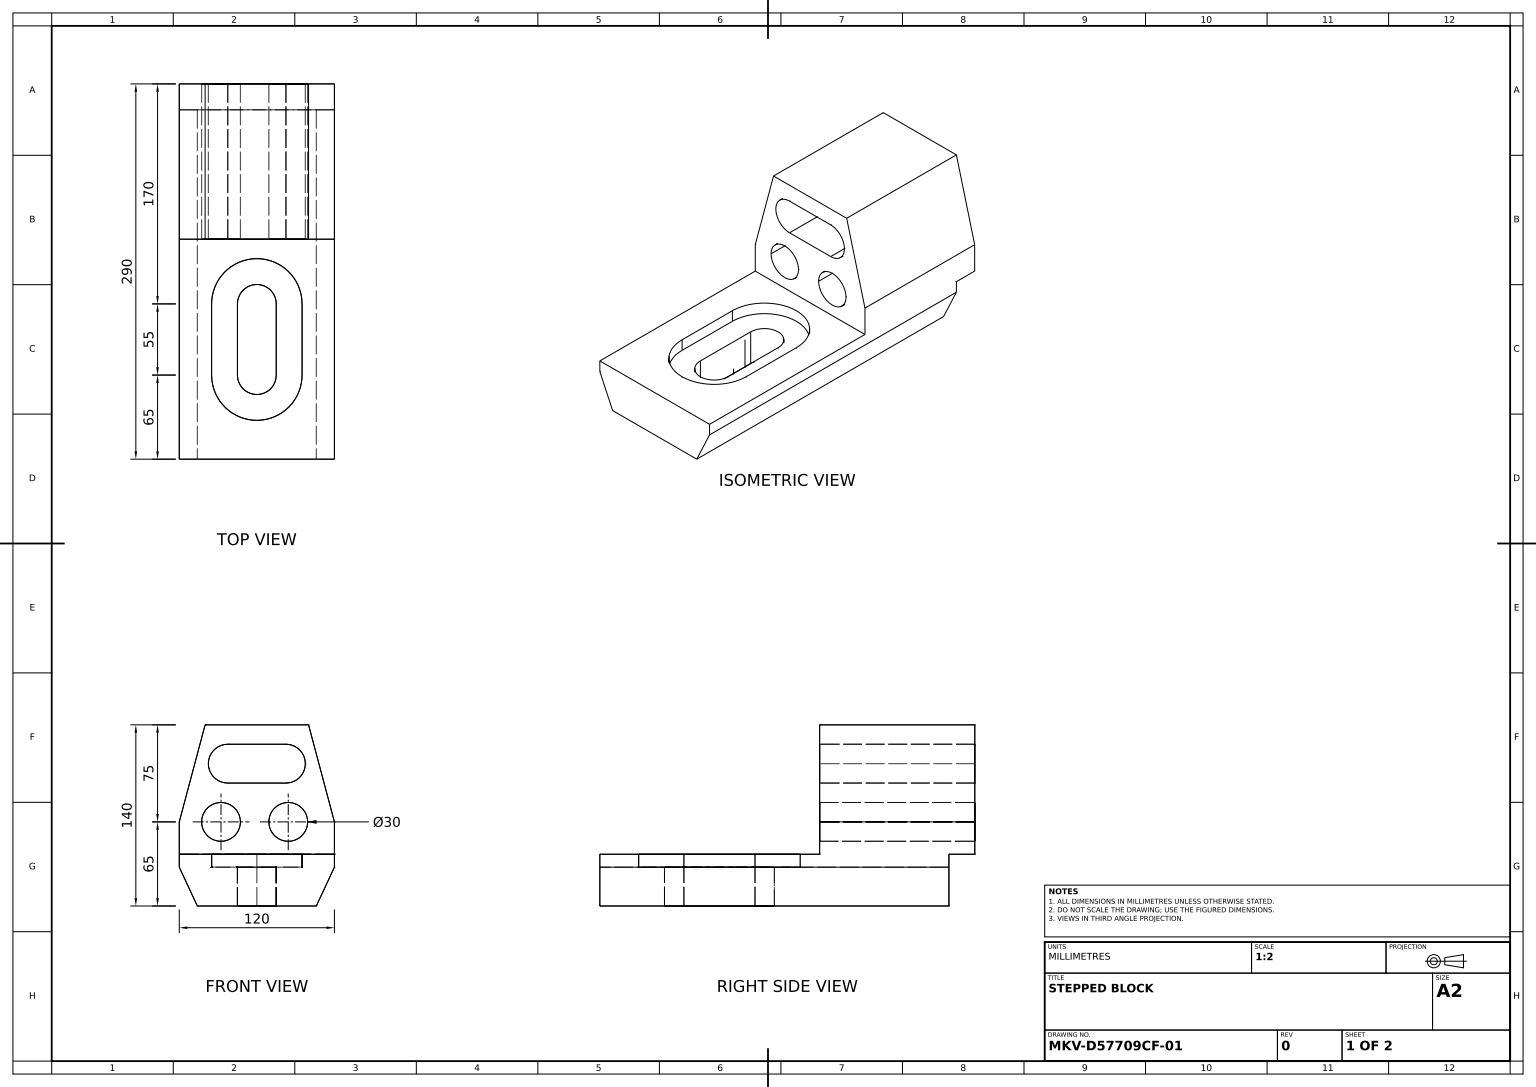
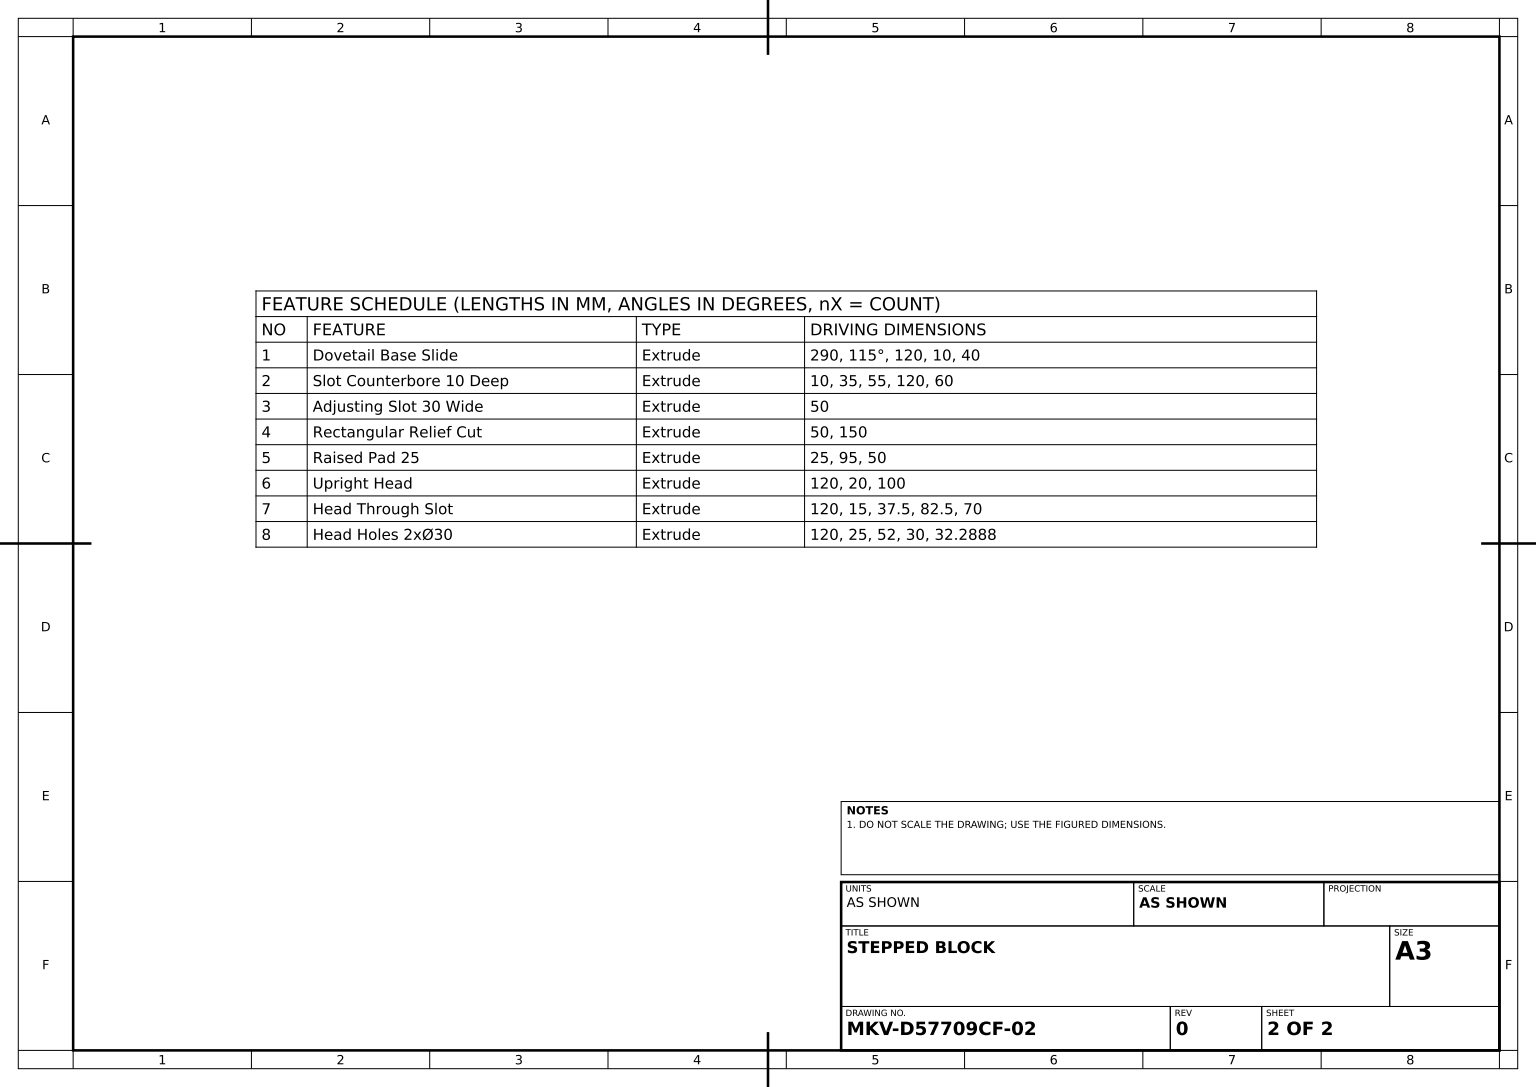
from build123d import *

# Parameters (mm, degrees)
DOVETAIL_BASE_SLIDE_DEPTH      = 290
SLOT_COUNTERBORE_10_DEEP_DEPTH = 10
ADJUSTING_SLOT_30_WIDE_DEPTH   = 50
RELIEF_CUT_SKETCH_W            = 120
RELIEF_CUT_SKETCH_H            = 20
RECTANGULAR_RELIEF_CUT_DEPTH   = 50
RAISED_PAD_SKETCH_W            = 120
RAISED_PAD_SKETCH_H            = 120
RAISED_PAD_25_DEPTH            = 25
UPRIGHT_HEAD_DEPTH             = 120
HEAD_THROUGH_SLOT_DEPTH        = 120
HEAD_HOLES_SKETCH_R            = 15
HEAD_HOLES_2X_30_DEPTH         = 120


with BuildPart() as part:
    # Dovetail Base Profile Sketch → Dovetail Base Slide (new body)
    with BuildSketch(Plane.XY):
        Polygon((106.010770255, 40), (106.010770255, 30), (92.021540511, 0), (0, 0), (-13.989229745, 30), (-13.989229745, 40), align=None)
    extrude(amount=-DOVETAIL_BASE_SLIDE_DEPTH)

    # Slot Counterbore Sketch → Slot Counterbore 10 Deep (cut)
    with BuildSketch(Plane(origin=(0, 40, 0), x_dir=(1, 0, 0), z_dir=(0, 1, 0))):
        with BuildLine():
            Line((11.010770255, 120), (11.010770255, 65))
            ThreePointArc((11.010770255, 65), (46.010770255, 30), (81.010770255, 65))
            Line((81.010770255, 65), (81.010770255, 120))
            ThreePointArc((81.010770255, 120), (46.010770255, 155), (11.010770255, 120))
        make_face()
    extrude(amount=-SLOT_COUNTERBORE_10_DEEP_DEPTH, mode=Mode.SUBTRACT)

    # Adjusting Slot Sketch → Adjusting Slot 30 Wide (cut)
    with BuildSketch(Plane(origin=(0, 30, 0), x_dir=(1, 0, 0), z_dir=(0, 1, 0))):
        with BuildLine():
            Line((31.010770255, 120), (31.010770255, 65))
            ThreePointArc((31.010770255, 65), (46.010770255, 50), (61.010770255, 65))
            Line((61.010770255, 65), (61.010770255, 120))
            ThreePointArc((61.010770255, 120), (46.010770255, 135), (31.010770255, 120))
        make_face()
    extrude(amount=-ADJUSTING_SLOT_30_WIDE_DEPTH, mode=Mode.SUBTRACT)

    # Relief Cut Sketch → Rectangular Relief Cut (cut)
    with BuildSketch(Plane(origin=(0, 40, 0), x_dir=(1, 0, 0), z_dir=(0, 1, 0))):
        with Locations((46.010770255, 280)):
            Rectangle(RELIEF_CUT_SKETCH_W, RELIEF_CUT_SKETCH_H)
    extrude(amount=-RECTANGULAR_RELIEF_CUT_DEPTH, mode=Mode.SUBTRACT)

    # Raised Pad Sketch → Raised Pad 25 (add)
    with BuildSketch(Plane(origin=(0, 40, 0), x_dir=(1, 0, 0), z_dir=(0, 1, 0))):
        with Locations((46.010770255, 230)):
            Rectangle(RAISED_PAD_SKETCH_W, RAISED_PAD_SKETCH_H)
    extrude(amount=RAISED_PAD_25_DEPTH)

    # Upright Head Profile Sketch → Upright Head (add)
    with BuildSketch(Plane.XY.offset(-170)):
        Polygon((46.010770255, 140), (6.010770255, 140), (-13.989229745, 65), (106.010770255, 65), (86.010770255, 140), align=None)
    extrude(amount=-UPRIGHT_HEAD_DEPTH)

    # Head Slot Sketch → Head Through Slot (cut)
    with BuildSketch(Plane.XY.offset(-170)):
        with BuildLine():
            Line((23.510770255, 125), (68.510770255, 125))
            ThreePointArc((68.510770255, 125), (83.510770255, 110), (68.510770255, 95))
            Line((68.510770255, 95), (23.510770255, 95))
            ThreePointArc((23.510770255, 95), (8.510770255, 110), (23.510770255, 125))
        make_face()
    extrude(amount=-HEAD_THROUGH_SLOT_DEPTH, mode=Mode.SUBTRACT)

    # Head Holes Sketch → Head Holes 2xØ30 (cut)
    with BuildSketch(Plane.XY.offset(-170)):
        with Locations((18.299617998, 65)):
            Circle(HEAD_HOLES_SKETCH_R)
        with Locations((70.299617998, 65)):
            Circle(HEAD_HOLES_SKETCH_R)
    extrude(amount=-HEAD_HOLES_2X_30_DEPTH, mode=Mode.SUBTRACT)


solid = part.part
